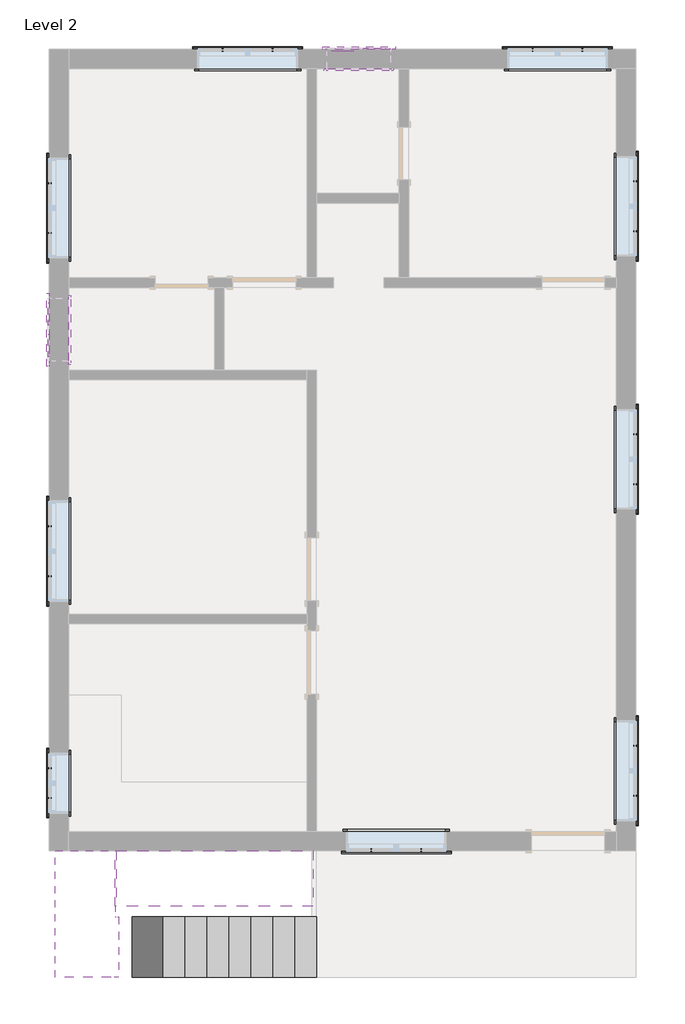
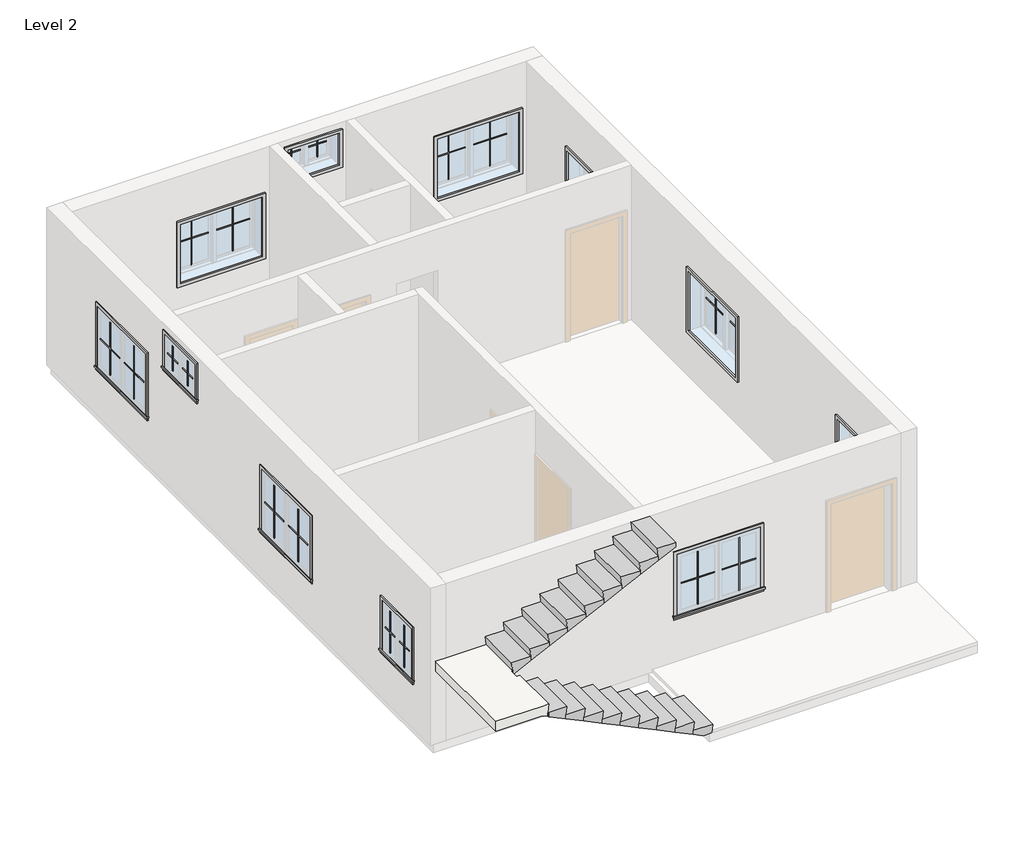
# One storey, part 2 of 2: 44 proxies, 2 stair flights, 1 slab.
"""IFC4 building model written with IfcOpenShell, lengths in millimetres."""

from ifc_helpers import new_model, si_unit, origin, place, context, project, spatial, faceted_brep, transform, mapped, element, save
from components import muntin_pattern_2x2_muntin_pattern_2x2_b3fe6957, muntin_pattern_2x2_muntin_pattern_2x2_3e0ecaf2, muntin_pattern_2x2_muntin_pattern_2x2_27d56209, muntin_pattern_2x2_muntin_pattern_2x2_bc89accc, muntin_pattern_2x2_muntin_pattern_2x2_1fe271a4, muntin_pattern_2x2_muntin_pattern_2x2_11ff06db, trim_window_exterior_flat_with_sill_41619996, trim_window_exterior_flat_with_sill_40e754a6, trim_window_exterior_flat_with_sill_f4abd27b, trim_window_interior_flat_picture_frame_51c85655, trim_window_interior_flat_picture_frame_6592d821, trim_window_interior_flat_picture_frame_286514af

model = new_model("IFC4")

# Units and contexts
model_context = context("Model", 3, world=origin())
ifc_project = project(units=[si_unit("LENGTHUNIT", "METRE", prefix="MILLI")], contexts=[model_context])

# Site, building, storey
site = spatial("IfcSite", under=ifc_project)
building = spatial("IfcBuilding", under=site)
storey = spatial("IfcBuildingStorey", under=building, Name="Level 2", Elevation=3048.0)

# Proxies
placement = place(None, origin())
muntin_pattern_2x2_muntin_pattern_2x2_shape = muntin_pattern_2x2_muntin_pattern_2x2_b3fe6957(model_context)
element("IfcBuildingElementProxy", 1, Name="Muntin Pattern_2x2 : Muntin Pattern_2x2", ObjectType="Muntin Pattern_2x2 : Muntin Pattern_2x2", at=placement, inside=storey, context=model_context, shape_type="MappedRepresentation", body=[
    mapped(muntin_pattern_2x2_muntin_pattern_2x2_shape, transform((-8839.6634077, -4303.4328663, 4032.25), x_axis=(0.0, 1.0, 0.0), y_axis=(-1.0, 0.0, 0.0), z_axis=(0.0, 0.0, 1.0))),
])
muntin_pattern_2x2_muntin_pattern_2x2_2_shape = muntin_pattern_2x2_muntin_pattern_2x2_3e0ecaf2(model_context)
element("IfcBuildingElementProxy", 2, Name="Muntin Pattern_2x2 : Muntin Pattern_2x2", ObjectType="Muntin Pattern_2x2 : Muntin Pattern_2x2", at=placement, inside=storey, context=model_context, shape_type="MappedRepresentation", body=[
    mapped(muntin_pattern_2x2_muntin_pattern_2x2_2_shape, transform((-8839.6634077, -3874.8078663, 4032.25), x_axis=(0.0, -1.0, 0.0), y_axis=(1.0, 0.0, 0.0), z_axis=(0.0, 0.0, 1.0))),
])
muntin_pattern_2x2_muntin_pattern_2x2_3_shape = muntin_pattern_2x2_muntin_pattern_2x2_27d56209(model_context)
element("IfcBuildingElementProxy", 3, Name="Muntin Pattern_2x2 : Muntin Pattern_2x2", ObjectType="Muntin Pattern_2x2 : Muntin Pattern_2x2", at=placement, inside=storey, context=model_context, shape_type="MappedRepresentation", body=[
    mapped(muntin_pattern_2x2_muntin_pattern_2x2_3_shape, transform((-8839.6634077, 2226.7657273, 5251.45), x_axis=(0.0, 1.0, 0.0), y_axis=(-1.0, 0.0, 0.0), z_axis=(0.0, 0.0, 1.0))),
])
element("IfcBuildingElementProxy", 4, Name="Muntin Pattern_2x2 : Muntin Pattern_2x2", ObjectType="Muntin Pattern_2x2 : Muntin Pattern_2x2", at=placement, inside=storey, context=model_context, shape_type="MappedRepresentation", body=[
    mapped(muntin_pattern_2x2_muntin_pattern_2x2_3_shape, transform((-4603.9220229, 6494.5392844, 5251.45), x_axis=(1.0, 0.0, 0.0), y_axis=(0.0, 1.0, 0.0), z_axis=(0.0, 0.0, 1.0))),
])
muntin_pattern_2x2_muntin_pattern_2x2_4_shape = muntin_pattern_2x2_muntin_pattern_2x2_bc89accc(model_context)
element("IfcBuildingElementProxy", 5, Name="Muntin Pattern_2x2 : Muntin Pattern_2x2", ObjectType="Muntin Pattern_2x2 : Muntin Pattern_2x2", at=placement, inside=storey, context=model_context, shape_type="MappedRepresentation", body=[
    mapped(muntin_pattern_2x2_muntin_pattern_2x2_4_shape, transform((-8839.6634077, 2680.7907273, 5251.45), x_axis=(0.0, -1.0, 0.0), y_axis=(1.0, 0.0, 0.0), z_axis=(0.0, 0.0, 1.0))),
])
element("IfcBuildingElementProxy", 6, Name="Muntin Pattern_2x2 : Muntin Pattern_2x2", ObjectType="Muntin Pattern_2x2 : Muntin Pattern_2x2", at=placement, inside=storey, context=model_context, shape_type="MappedRepresentation", body=[
    mapped(muntin_pattern_2x2_muntin_pattern_2x2_4_shape, transform((-4149.8970229, 6494.5392844, 5251.45), x_axis=(-1.0, 0.0, 0.0), y_axis=(0.0, -1.0, 0.0), z_axis=(0.0, 0.0, 1.0))),
])
muntin_pattern_2x2_muntin_pattern_2x2_5_shape = muntin_pattern_2x2_muntin_pattern_2x2_1fe271a4(model_context)
element("IfcBuildingElementProxy", 7, Name="Muntin Pattern_2x2 : Muntin Pattern_2x2", ObjectType="Muntin Pattern_2x2 : Muntin Pattern_2x2", at=placement, inside=storey, context=model_context, shape_type="MappedRepresentation", body=[
    mapped(muntin_pattern_2x2_muntin_pattern_2x2_5_shape, transform((-385.3035282, -3550.9578663, 4032.25), x_axis=(0.0, -1.0, 0.0), y_axis=(1.0, 0.0, 0.0), z_axis=(0.0, 0.0, 1.0))),
])
element("IfcBuildingElementProxy", 8, Name="Muntin Pattern_2x2 : Muntin Pattern_2x2", ObjectType="Muntin Pattern_2x2 : Muntin Pattern_2x2", at=placement, inside=storey, context=model_context, shape_type="MappedRepresentation", body=[
    mapped(muntin_pattern_2x2_muntin_pattern_2x2_5_shape, transform((-385.3035282, 944.8421337, 4032.25), x_axis=(0.0, -1.0, 0.0), y_axis=(1.0, 0.0, 0.0), z_axis=(0.0, 0.0, 1.0))),
])
element("IfcBuildingElementProxy", 9, Name="Muntin Pattern_2x2 : Muntin Pattern_2x2", ObjectType="Muntin Pattern_2x2 : Muntin Pattern_2x2", at=placement, inside=storey, context=model_context, shape_type="MappedRepresentation", body=[
    mapped(muntin_pattern_2x2_muntin_pattern_2x2_5_shape, transform((-385.3035282, 4597.1928819, 4032.25), x_axis=(0.0, -1.0, 0.0), y_axis=(1.0, 0.0, 0.0), z_axis=(0.0, 0.0, 1.0))),
])
element("IfcBuildingElementProxy", 10, Name="Muntin Pattern_2x2 : Muntin Pattern_2x2", ObjectType="Muntin Pattern_2x2 : Muntin Pattern_2x2", at=placement, inside=storey, context=model_context, shape_type="MappedRepresentation", body=[
    mapped(muntin_pattern_2x2_muntin_pattern_2x2_5_shape, transform((-1866.4410282, 6494.5392844, 4032.25), x_axis=(1.0, 0.0, 0.0), y_axis=(0.0, 1.0, 0.0), z_axis=(0.0, 0.0, 1.0))),
])
element("IfcBuildingElementProxy", 11, Name="Muntin Pattern_2x2 : Muntin Pattern_2x2", ObjectType="Muntin Pattern_2x2 : Muntin Pattern_2x2", at=placement, inside=storey, context=model_context, shape_type="MappedRepresentation", body=[
    mapped(muntin_pattern_2x2_muntin_pattern_2x2_5_shape, transform((-6342.5074828, 6494.5392844, 4032.25), x_axis=(1.0, 0.0, 0.0), y_axis=(0.0, 1.0, 0.0), z_axis=(0.0, 0.0, 1.0))),
])
element("IfcBuildingElementProxy", 12, Name="Muntin Pattern_2x2 : Muntin Pattern_2x2", ObjectType="Muntin Pattern_2x2 : Muntin Pattern_2x2", at=placement, inside=storey, context=model_context, shape_type="MappedRepresentation", body=[
    mapped(muntin_pattern_2x2_muntin_pattern_2x2_5_shape, transform((-8839.6634077, 3851.0678819, 4032.25), x_axis=(0.0, 1.0, 0.0), y_axis=(-1.0, 0.0, 0.0), z_axis=(0.0, 0.0, 1.0))),
])
element("IfcBuildingElementProxy", 13, Name="Muntin Pattern_2x2 : Muntin Pattern_2x2", ObjectType="Muntin Pattern_2x2 : Muntin Pattern_2x2", at=placement, inside=storey, context=model_context, shape_type="MappedRepresentation", body=[
    mapped(muntin_pattern_2x2_muntin_pattern_2x2_5_shape, transform((-8839.6634077, -1101.0873314, 4032.25), x_axis=(0.0, 1.0, 0.0), y_axis=(-1.0, 0.0, 0.0), z_axis=(0.0, 0.0, 1.0))),
])
element("IfcBuildingElementProxy", 14, Name="Muntin Pattern_2x2 : Muntin Pattern_2x2", ObjectType="Muntin Pattern_2x2 : Muntin Pattern_2x2", at=placement, inside=storey, context=model_context, shape_type="MappedRepresentation", body=[
    mapped(muntin_pattern_2x2_muntin_pattern_2x2_5_shape, transform((-3475.4824828, -5057.4953663, 4032.25), x_axis=(-1.0, 0.0, 0.0), y_axis=(0.0, -1.0, 0.0), z_axis=(0.0, 0.0, 1.0))),
])
muntin_pattern_2x2_muntin_pattern_2x2_6_shape = muntin_pattern_2x2_muntin_pattern_2x2_11ff06db(model_context)
element("IfcBuildingElementProxy", 15, Name="Muntin Pattern_2x2 : Muntin Pattern_2x2", ObjectType="Muntin Pattern_2x2 : Muntin Pattern_2x2", at=placement, inside=storey, context=model_context, shape_type="MappedRepresentation", body=[
    mapped(muntin_pattern_2x2_muntin_pattern_2x2_6_shape, transform((-385.3035282, -4271.6828663, 4032.25), x_axis=(0.0, 1.0, 0.0), y_axis=(-1.0, 0.0, 0.0), z_axis=(0.0, 0.0, 1.0))),
])
element("IfcBuildingElementProxy", 16, Name="Muntin Pattern_2x2 : Muntin Pattern_2x2", ObjectType="Muntin Pattern_2x2 : Muntin Pattern_2x2", at=placement, inside=storey, context=model_context, shape_type="MappedRepresentation", body=[
    mapped(muntin_pattern_2x2_muntin_pattern_2x2_6_shape, transform((-385.3035282, 224.1171337, 4032.25), x_axis=(0.0, 1.0, 0.0), y_axis=(-1.0, 0.0, 0.0), z_axis=(0.0, 0.0, 1.0))),
])
element("IfcBuildingElementProxy", 17, Name="Muntin Pattern_2x2 : Muntin Pattern_2x2", ObjectType="Muntin Pattern_2x2 : Muntin Pattern_2x2", at=placement, inside=storey, context=model_context, shape_type="MappedRepresentation", body=[
    mapped(muntin_pattern_2x2_muntin_pattern_2x2_6_shape, transform((-385.3035282, 3876.4678819, 4032.25), x_axis=(0.0, 1.0, 0.0), y_axis=(-1.0, 0.0, 0.0), z_axis=(0.0, 0.0, 1.0))),
])
element("IfcBuildingElementProxy", 18, Name="Muntin Pattern_2x2 : Muntin Pattern_2x2", ObjectType="Muntin Pattern_2x2 : Muntin Pattern_2x2", at=placement, inside=storey, context=model_context, shape_type="MappedRepresentation", body=[
    mapped(muntin_pattern_2x2_muntin_pattern_2x2_6_shape, transform((-1145.7160282, 6494.5392844, 4032.25), x_axis=(-1.0, 0.0, 0.0), y_axis=(0.0, -1.0, 0.0), z_axis=(0.0, 0.0, 1.0))),
])
element("IfcBuildingElementProxy", 19, Name="Muntin Pattern_2x2 : Muntin Pattern_2x2", ObjectType="Muntin Pattern_2x2 : Muntin Pattern_2x2", at=placement, inside=storey, context=model_context, shape_type="MappedRepresentation", body=[
    mapped(muntin_pattern_2x2_muntin_pattern_2x2_6_shape, transform((-5621.7824828, 6494.5392844, 4032.25), x_axis=(-1.0, 0.0, 0.0), y_axis=(0.0, -1.0, 0.0), z_axis=(0.0, 0.0, 1.0))),
])
element("IfcBuildingElementProxy", 20, Name="Muntin Pattern_2x2 : Muntin Pattern_2x2", ObjectType="Muntin Pattern_2x2 : Muntin Pattern_2x2", at=placement, inside=storey, context=model_context, shape_type="MappedRepresentation", body=[
    mapped(muntin_pattern_2x2_muntin_pattern_2x2_6_shape, transform((-8839.6634077, 4571.7928819, 4032.25), x_axis=(0.0, -1.0, 0.0), y_axis=(1.0, 0.0, 0.0), z_axis=(0.0, 0.0, 1.0))),
])
element("IfcBuildingElementProxy", 21, Name="Muntin Pattern_2x2 : Muntin Pattern_2x2", ObjectType="Muntin Pattern_2x2 : Muntin Pattern_2x2", at=placement, inside=storey, context=model_context, shape_type="MappedRepresentation", body=[
    mapped(muntin_pattern_2x2_muntin_pattern_2x2_6_shape, transform((-8839.6634077, -380.3623314, 4032.25), x_axis=(0.0, -1.0, 0.0), y_axis=(1.0, 0.0, 0.0), z_axis=(0.0, 0.0, 1.0))),
])
element("IfcBuildingElementProxy", 22, Name="Muntin Pattern_2x2 : Muntin Pattern_2x2", ObjectType="Muntin Pattern_2x2 : Muntin Pattern_2x2", at=placement, inside=storey, context=model_context, shape_type="MappedRepresentation", body=[
    mapped(muntin_pattern_2x2_muntin_pattern_2x2_6_shape, transform((-4196.2074828, -5057.4953663, 4032.25), x_axis=(1.0, 0.0, 0.0), y_axis=(0.0, 1.0, 0.0), z_axis=(0.0, 0.0, 1.0))),
])
trim_window_exterior_flat_with_sill_shape = trim_window_exterior_flat_with_sill_41619996(model_context)
element("IfcBuildingElementProxy", 23, Name="Trim-Window-Exterior-Flat : with Sill", ObjectType="Trim-Window-Exterior-Flat : with Sill", at=placement, inside=storey, context=model_context, shape_type="MappedRepresentation", body=[
    mapped(trim_window_exterior_flat_with_sill_shape, transform((-8849.1884077, -4089.1203663, 4876.8), x_axis=(0.0, -1.0, 0.0), y_axis=(0.0, 0.0, 1.0), z_axis=(-1.0, 0.0, 0.0))),
])
trim_window_exterior_flat_with_sill_2_shape = trim_window_exterior_flat_with_sill_40e754a6(model_context)
element("IfcBuildingElementProxy", 24, Name="Trim-Window-Exterior-Flat : with Sill", ObjectType="Trim-Window-Exterior-Flat : with Sill", at=placement, inside=storey, context=model_context, shape_type="MappedRepresentation", body=[
    mapped(trim_window_exterior_flat_with_sill_2_shape, transform((-8849.1884077, 2453.7782273, 5791.2), x_axis=(0.0, -1.0, 0.0), y_axis=(0.0, 0.0, 1.0), z_axis=(-1.0, 0.0, 0.0))),
])
element("IfcBuildingElementProxy", 25, Name="Trim-Window-Exterior-Flat : with Sill", ObjectType="Trim-Window-Exterior-Flat : with Sill", at=placement, inside=storey, context=model_context, shape_type="MappedRepresentation", body=[
    mapped(trim_window_exterior_flat_with_sill_2_shape, transform((-4376.9095229, 6504.0642844, 5791.2), x_axis=(-1.0, 0.0, 0.0), y_axis=(0.0, 0.0, 1.0), z_axis=(0.0, 1.0, 0.0))),
])
trim_window_exterior_flat_with_sill_3_shape = trim_window_exterior_flat_with_sill_f4abd27b(model_context)
element("IfcBuildingElementProxy", 26, Name="Trim-Window-Exterior-Flat : with Sill", ObjectType="Trim-Window-Exterior-Flat : with Sill", at=placement, inside=storey, context=model_context, shape_type="MappedRepresentation", body=[
    mapped(trim_window_exterior_flat_with_sill_3_shape, transform((-375.7785282, -3911.3203663, 5080.0), x_axis=(0.0, 1.0, 0.0), y_axis=(0.0, 0.0, 1.0), z_axis=(1.0, 0.0, 0.0))),
])
element("IfcBuildingElementProxy", 27, Name="Trim-Window-Exterior-Flat : with Sill", ObjectType="Trim-Window-Exterior-Flat : with Sill", at=placement, inside=storey, context=model_context, shape_type="MappedRepresentation", body=[
    mapped(trim_window_exterior_flat_with_sill_3_shape, transform((-375.7785282, 584.4796337, 5080.0), x_axis=(0.0, 1.0, 0.0), y_axis=(0.0, 0.0, 1.0), z_axis=(1.0, 0.0, 0.0))),
])
element("IfcBuildingElementProxy", 28, Name="Trim-Window-Exterior-Flat : with Sill", ObjectType="Trim-Window-Exterior-Flat : with Sill", at=placement, inside=storey, context=model_context, shape_type="MappedRepresentation", body=[
    mapped(trim_window_exterior_flat_with_sill_3_shape, transform((-375.7785282, 4236.8303819, 5080.0), x_axis=(0.0, 1.0, 0.0), y_axis=(0.0, 0.0, 1.0), z_axis=(1.0, 0.0, 0.0))),
])
element("IfcBuildingElementProxy", 29, Name="Trim-Window-Exterior-Flat : with Sill", ObjectType="Trim-Window-Exterior-Flat : with Sill", at=placement, inside=storey, context=model_context, shape_type="MappedRepresentation", body=[
    mapped(trim_window_exterior_flat_with_sill_3_shape, transform((-1506.0785282, 6504.0642844, 5080.0), x_axis=(-1.0, 0.0, 0.0), y_axis=(0.0, 0.0, 1.0), z_axis=(0.0, 1.0, 0.0))),
])
element("IfcBuildingElementProxy", 30, Name="Trim-Window-Exterior-Flat : with Sill", ObjectType="Trim-Window-Exterior-Flat : with Sill", at=placement, inside=storey, context=model_context, shape_type="MappedRepresentation", body=[
    mapped(trim_window_exterior_flat_with_sill_3_shape, transform((-5982.1449828, 6504.0642844, 5080.0), x_axis=(-1.0, 0.0, 0.0), y_axis=(0.0, 0.0, 1.0), z_axis=(0.0, 1.0, 0.0))),
])
element("IfcBuildingElementProxy", 31, Name="Trim-Window-Exterior-Flat : with Sill", ObjectType="Trim-Window-Exterior-Flat : with Sill", at=placement, inside=storey, context=model_context, shape_type="MappedRepresentation", body=[
    mapped(trim_window_exterior_flat_with_sill_3_shape, transform((-8849.1884077, 4211.4303819, 5080.0), x_axis=(0.0, -1.0, 0.0), y_axis=(0.0, 0.0, 1.0), z_axis=(-1.0, 0.0, 0.0))),
])
element("IfcBuildingElementProxy", 32, Name="Trim-Window-Exterior-Flat : with Sill", ObjectType="Trim-Window-Exterior-Flat : with Sill", at=placement, inside=storey, context=model_context, shape_type="MappedRepresentation", body=[
    mapped(trim_window_exterior_flat_with_sill_3_shape, transform((-8849.1884077, -740.7248314, 5080.0), x_axis=(0.0, -1.0, 0.0), y_axis=(0.0, 0.0, 1.0), z_axis=(-1.0, 0.0, 0.0))),
])
element("IfcBuildingElementProxy", 33, Name="Trim-Window-Exterior-Flat : with Sill", ObjectType="Trim-Window-Exterior-Flat : with Sill", at=placement, inside=storey, context=model_context, shape_type="MappedRepresentation", body=[
    mapped(trim_window_exterior_flat_with_sill_3_shape, transform((-3835.8449828, -5067.0203663, 5080.0), x_axis=(1.0, 0.0, 0.0), y_axis=(0.0, 0.0, 1.0), z_axis=(0.0, -1.0, 0.0))),
])
trim_window_interior_flat_picture_frame_shape = trim_window_interior_flat_picture_frame_51c85655(model_context)
element("IfcBuildingElementProxy", 34, Name="Trim-Window-Interior-Flat : Picture Frame", ObjectType="Trim-Window-Interior-Flat : Picture Frame", at=placement, inside=storey, context=model_context, shape_type="MappedRepresentation", body=[
    mapped(trim_window_interior_flat_picture_frame_shape, transform((-8569.7884077, -4089.1203663, 4876.8), x_axis=(0.0, 1.0, 0.0), y_axis=(0.0, 0.0, 1.0), z_axis=(1.0, 0.0, 0.0))),
])
trim_window_interior_flat_picture_frame_2_shape = trim_window_interior_flat_picture_frame_6592d821(model_context)
element("IfcBuildingElementProxy", 35, Name="Trim-Window-Interior-Flat : Picture Frame", ObjectType="Trim-Window-Interior-Flat : Picture Frame", at=placement, inside=storey, context=model_context, shape_type="MappedRepresentation", body=[
    mapped(trim_window_interior_flat_picture_frame_2_shape, transform((-8569.7884077, 2453.7782273, 5791.2), x_axis=(0.0, 1.0, 0.0), y_axis=(0.0, 0.0, 1.0), z_axis=(1.0, 0.0, 0.0))),
])
element("IfcBuildingElementProxy", 36, Name="Trim-Window-Interior-Flat : Picture Frame", ObjectType="Trim-Window-Interior-Flat : Picture Frame", at=placement, inside=storey, context=model_context, shape_type="MappedRepresentation", body=[
    mapped(trim_window_interior_flat_picture_frame_2_shape, transform((-4376.9095229, 6224.6642844, 5791.2), x_axis=(1.0, 0.0, 0.0), y_axis=(0.0, 0.0, 1.0), z_axis=(0.0, -1.0, 0.0))),
])
trim_window_interior_flat_picture_frame_3_shape = trim_window_interior_flat_picture_frame_286514af(model_context)
element("IfcBuildingElementProxy", 37, Name="Trim-Window-Interior-Flat : Picture Frame", ObjectType="Trim-Window-Interior-Flat : Picture Frame", at=placement, inside=storey, context=model_context, shape_type="MappedRepresentation", body=[
    mapped(trim_window_interior_flat_picture_frame_3_shape, transform((-655.1785282, -3911.3203663, 5080.0), x_axis=(0.0, -1.0, 0.0), y_axis=(0.0, 0.0, 1.0), z_axis=(-1.0, 0.0, 0.0))),
])
element("IfcBuildingElementProxy", 38, Name="Trim-Window-Interior-Flat : Picture Frame", ObjectType="Trim-Window-Interior-Flat : Picture Frame", at=placement, inside=storey, context=model_context, shape_type="MappedRepresentation", body=[
    mapped(trim_window_interior_flat_picture_frame_3_shape, transform((-655.1785282, 584.4796337, 5080.0), x_axis=(0.0, -1.0, 0.0), y_axis=(0.0, 0.0, 1.0), z_axis=(-1.0, 0.0, 0.0))),
])
element("IfcBuildingElementProxy", 39, Name="Trim-Window-Interior-Flat : Picture Frame", ObjectType="Trim-Window-Interior-Flat : Picture Frame", at=placement, inside=storey, context=model_context, shape_type="MappedRepresentation", body=[
    mapped(trim_window_interior_flat_picture_frame_3_shape, transform((-655.1785282, 4236.8303819, 5080.0), x_axis=(0.0, -1.0, 0.0), y_axis=(0.0, 0.0, 1.0), z_axis=(-1.0, 0.0, 0.0))),
])
element("IfcBuildingElementProxy", 40, Name="Trim-Window-Interior-Flat : Picture Frame", ObjectType="Trim-Window-Interior-Flat : Picture Frame", at=placement, inside=storey, context=model_context, shape_type="MappedRepresentation", body=[
    mapped(trim_window_interior_flat_picture_frame_3_shape, transform((-1506.0785282, 6224.6642844, 5080.0), x_axis=(1.0, 0.0, 0.0), y_axis=(0.0, 0.0, 1.0), z_axis=(0.0, -1.0, 0.0))),
])
element("IfcBuildingElementProxy", 41, Name="Trim-Window-Interior-Flat : Picture Frame", ObjectType="Trim-Window-Interior-Flat : Picture Frame", at=placement, inside=storey, context=model_context, shape_type="MappedRepresentation", body=[
    mapped(trim_window_interior_flat_picture_frame_3_shape, transform((-5982.1449828, 6224.6642844, 5080.0), x_axis=(1.0, 0.0, 0.0), y_axis=(0.0, 0.0, 1.0), z_axis=(0.0, -1.0, 0.0))),
])
element("IfcBuildingElementProxy", 42, Name="Trim-Window-Interior-Flat : Picture Frame", ObjectType="Trim-Window-Interior-Flat : Picture Frame", at=placement, inside=storey, context=model_context, shape_type="MappedRepresentation", body=[
    mapped(trim_window_interior_flat_picture_frame_3_shape, transform((-8569.7884077, 4211.4303819, 5080.0), x_axis=(0.0, 1.0, 0.0), y_axis=(0.0, 0.0, 1.0), z_axis=(1.0, 0.0, 0.0))),
])
element("IfcBuildingElementProxy", 43, Name="Trim-Window-Interior-Flat : Picture Frame", ObjectType="Trim-Window-Interior-Flat : Picture Frame", at=placement, inside=storey, context=model_context, shape_type="MappedRepresentation", body=[
    mapped(trim_window_interior_flat_picture_frame_3_shape, transform((-8569.7884077, -740.7248314, 5080.0), x_axis=(0.0, 1.0, 0.0), y_axis=(0.0, 0.0, 1.0), z_axis=(1.0, 0.0, 0.0))),
])
element("IfcBuildingElementProxy", 44, Name="Trim-Window-Interior-Flat : Picture Frame", ObjectType="Trim-Window-Interior-Flat : Picture Frame", at=placement, inside=storey, context=model_context, shape_type="MappedRepresentation", body=[
    mapped(trim_window_interior_flat_picture_frame_3_shape, transform((-3835.8449828, -4787.6203663, 5080.0), x_axis=(-1.0, 0.0, 0.0), y_axis=(0.0, 0.0, 1.0), z_axis=(0.0, 1.0, 0.0))),
])

# Slab
element("IfcSlab", 45, ObjectType="7\" Thickness", at=placement, inside=storey, context=model_context, shape_type="Brep", body=[
    faceted_brep([(-7896.6884077, -6018.2039507, 4572.0), (-7896.6884077, -5868.2058051, 4572.0), (-7877.6384077, -5868.2058051, 4572.0), (-7877.6384077, -5067.0203663, 4572.0), (-7896.6884077, -5067.0203663, 4572.0), (-8101.3126638, -5067.0203663, 4572.0), (-8760.2884077, -5067.0203663, 4572.0), (-8760.2884077, -6894.0922127, 4572.0), (-7955.5707267, -6894.0922127, 4572.0), (-7842.6949828, -6894.0922127, 4572.0), (-7842.6949828, -6018.2039507, 4572.0), (-7861.7449828, -6018.2039507, 4419.6), (-7861.7449828, -6894.0922127, 4419.6), (-7861.7449828, -6894.0922127, 4349.1636429), (-7861.7449828, -6018.2039507, 4349.1636429), (-7955.5707267, -6018.2039507, 4394.2), (-7896.6884077, -6018.2039507, 4394.2), (-7896.6884077, -5868.2058051, 4394.2), (-7896.6884077, -5868.2058051, 4492.4196429), (-7877.6384077, -5868.2058051, 4501.5636429), (-7877.6384077, -5067.0203663, 4501.5636429), (-7896.6884077, -5067.0203663, 4492.4196429), (-8101.3126638, -5067.0203663, 4394.2), (-8760.2884077, -5067.0203663, 4394.2), (-8760.2884077, -6894.0922127, 4394.2), (-7955.5707267, -6894.0922127, 4394.2), (-8101.3126638, -5868.2058051, 4394.2)], [[[0, 1, 2, 3, 4, 5, 6, 7, 8, 9, 10]], [[11, 12, 13, 14]], [[0, 10, 11, 14, 15, 16]], [[1, 0, 16, 17, 18]], [[2, 1, 18, 19]], [[3, 2, 19, 20]], [[4, 3, 20, 21]], [[4, 21, 22, 23, 6, 5]], [[7, 6, 23, 24]], [[12, 9, 8, 7, 24, 25, 13]], [[10, 9, 12, 11]], [[26, 17, 16, 15, 25, 24, 23, 22]], [[17, 26, 18]], [[25, 15, 14, 13]], [[26, 22, 21, 20, 19, 18]]]),
])

# Stair flights
element("IfcStairFlight", 46, ObjectType="3/4\" Nosing", at=placement, inside=storey, context=model_context, shape_type="Brep", body=[
    faceted_brep([(-4985.1949828, -6894.0922127, 3200.4), (-4985.1949828, -6018.2039507, 3200.4), (-5321.7449828, -6018.2039507, 3200.4), (-5321.7449828, -6894.0922127, 3200.4), (-5321.7449828, -6894.0922127, 3129.9636429), (-5150.9873934, -6894.0922127, 3048.0), (-5004.2449828, -6894.0922127, 3048.0), (-5004.2449828, -6018.2039507, 3048.0), (-5150.9873934, -6018.2039507, 3048.0), (-5321.7449828, -6018.2039507, 3129.9636429), (-5302.6949828, -6894.0922127, 3352.8), (-5302.6949828, -6018.2039507, 3352.8), (-5639.2449828, -6018.2039507, 3352.8), (-5639.2449828, -6894.0922127, 3352.8), (-5639.2449828, -6894.0922127, 3282.3636429), (-5639.2449828, -6018.2039507, 3282.3636429), (-5620.1949828, -6894.0922127, 3505.2), (-5620.1949828, -6018.2039507, 3505.2), (-5956.7449828, -6018.2039507, 3505.2), (-5956.7449828, -6894.0922127, 3505.2), (-5956.7449828, -6894.0922127, 3434.7636429), (-5956.7449828, -6018.2039507, 3434.7636429), (-5937.6949828, -6894.0922127, 3657.6), (-5937.6949828, -6018.2039507, 3657.6), (-6274.2449828, -6018.2039507, 3657.6), (-6274.2449828, -6894.0922127, 3657.6), (-6274.2449828, -6894.0922127, 3587.1636429), (-6274.2449828, -6018.2039507, 3587.1636429), (-6255.1949828, -6894.0922127, 3810.0), (-6255.1949828, -6018.2039507, 3810.0), (-6591.7449828, -6018.2039507, 3810.0), (-6591.7449828, -6894.0922127, 3810.0), (-6591.7449828, -6894.0922127, 3739.5636429), (-6591.7449828, -6018.2039507, 3739.5636429), (-6572.6949828, -6894.0922127, 3962.4), (-6572.6949828, -6018.2039507, 3962.4), (-6909.2449828, -6018.2039507, 3962.4), (-6909.2449828, -6894.0922127, 3962.4), (-6909.2449828, -6894.0922127, 3891.9636429), (-6909.2449828, -6018.2039507, 3891.9636429), (-6890.1949828, -6894.0922127, 4114.8), (-6890.1949828, -6018.2039507, 4114.8), (-7226.7449828, -6018.2039507, 4114.8), (-7226.7449828, -6894.0922127, 4114.8), (-7226.7449828, -6894.0922127, 4044.3636429), (-7226.7449828, -6018.2039507, 4044.3636429), (-7207.6949828, -6894.0922127, 4267.2), (-7207.6949828, -6018.2039507, 4267.2), (-7544.2449828, -6018.2039507, 4267.2), (-7544.2449828, -6894.0922127, 4267.2), (-7544.2449828, -6894.0922127, 4196.7636429), (-7544.2449828, -6018.2039507, 4196.7636429), (-7861.7449828, -6894.0922127, 4419.6), (-7842.6949828, -6894.0922127, 4419.6), (-7525.1949828, -6894.0922127, 4419.6), (-7525.1949828, -6018.2039507, 4419.6), (-7842.6949828, -6018.2039507, 4419.6), (-7861.7449828, -6018.2039507, 4419.6), (-7861.7449828, -6894.0922127, 4349.1636429), (-7842.6949828, -6894.0922127, 4340.0196429), (-7842.6949828, -6018.2039507, 4340.0196429), (-7861.7449828, -6018.2039507, 4349.1636429)], [[[0, 1, 2, 3]], [[0, 3, 4, 5, 6]], [[2, 1, 7, 8, 9]], [[10, 11, 12, 13]], [[10, 13, 14, 4, 3]], [[12, 11, 2, 9, 15]], [[16, 17, 18, 19]], [[16, 19, 20, 14, 13]], [[18, 17, 12, 15, 21]], [[22, 23, 24, 25]], [[22, 25, 26, 20, 19]], [[24, 23, 18, 21, 27]], [[28, 29, 30, 31]], [[28, 31, 32, 26, 25]], [[30, 29, 24, 27, 33]], [[34, 35, 36, 37]], [[34, 37, 38, 32, 31]], [[36, 35, 30, 33, 39]], [[40, 41, 42, 43]], [[40, 43, 44, 38, 37]], [[42, 41, 36, 39, 45]], [[46, 47, 48, 49]], [[46, 49, 50, 44, 43]], [[48, 47, 42, 45, 51]], [[52, 53, 54, 55, 56, 57]], [[53, 52, 58, 59]], [[54, 53, 59, 50, 49]], [[56, 55, 48, 51, 60]], [[57, 56, 60, 61]], [[52, 57, 61, 58]], [[1, 0, 6, 7]], [[3, 2, 11, 10]], [[13, 12, 17, 16]], [[19, 18, 23, 22]], [[25, 24, 29, 28]], [[31, 30, 35, 34]], [[37, 36, 41, 40]], [[43, 42, 47, 46]], [[49, 48, 55, 54]], [[7, 6, 5, 8]], [[8, 5, 4, 14, 20, 26, 32, 38, 44, 50, 59, 58, 61, 60, 51, 45, 39, 33, 27, 21, 15, 9]]]),
])
element("IfcStairFlight", 47, ObjectType="3/4\" Nosing", at=placement, inside=storey, context=model_context, shape_type="Brep", body=[
    faceted_brep([(-7896.6884077, -5067.0203663, 4724.4), (-7896.6884077, -5868.2058051, 4724.4), (-7560.1384077, -5868.2058051, 4724.4), (-7560.1384077, -5067.0203663, 4724.4), (-7560.1384077, -5067.0203663, 4653.9636429), (-7877.6384077, -5067.0203663, 4501.5636429), (-7877.6384077, -5067.0203663, 4572.0), (-7877.6384077, -5868.2058051, 4572.0), (-7877.6384077, -5868.2058051, 4501.5636429), (-7560.1384077, -5868.2058051, 4653.9636429), (-7579.1884077, -5067.0203663, 4876.8), (-7579.1884077, -5868.2058051, 4876.8), (-7242.6384077, -5868.2058051, 4876.8), (-7242.6384077, -5067.0203663, 4876.8), (-7242.6384077, -5067.0203663, 4806.3636429), (-7242.6384077, -5868.2058051, 4806.3636429), (-7261.6884077, -5067.0203663, 5029.2), (-7261.6884077, -5868.2058051, 5029.2), (-6925.1384077, -5868.2058051, 5029.2), (-6925.1384077, -5067.0203663, 5029.2), (-6925.1384077, -5067.0203663, 4958.7636429), (-6925.1384077, -5868.2058051, 4958.7636429), (-6944.1884077, -5067.0203663, 5181.6), (-6944.1884077, -5868.2058051, 5181.6), (-6607.6384077, -5868.2058051, 5181.6), (-6607.6384077, -5067.0203663, 5181.6), (-6607.6384077, -5067.0203663, 5111.1636429), (-6607.6384077, -5868.2058051, 5111.1636429), (-6626.6884077, -5067.0203663, 5334.0), (-6626.6884077, -5868.2058051, 5334.0), (-6290.1384077, -5868.2058051, 5334.0), (-6290.1384077, -5067.0203663, 5334.0), (-6290.1384077, -5067.0203663, 5263.5636429), (-6290.1384077, -5868.2058051, 5263.5636429), (-6309.1884077, -5067.0203663, 5486.4), (-6309.1884077, -5868.2058051, 5486.4), (-5972.6384077, -5868.2058051, 5486.4), (-5972.6384077, -5067.0203663, 5486.4), (-5972.6384077, -5067.0203663, 5415.9636429), (-5972.6384077, -5868.2058051, 5415.9636429), (-5991.6884077, -5067.0203663, 5638.8), (-5991.6884077, -5868.2058051, 5638.8), (-5655.1384077, -5868.2058051, 5638.8), (-5655.1384077, -5067.0203663, 5638.8), (-5655.1384077, -5067.0203663, 5568.3636429), (-5655.1384077, -5868.2058051, 5568.3636429), (-5674.1884077, -5067.0203663, 5791.2), (-5674.1884077, -5868.2058051, 5791.2), (-5337.6384077, -5868.2058051, 5791.2), (-5337.6384077, -5067.0203663, 5791.2), (-5337.6384077, -5067.0203663, 5720.7636429), (-5337.6384077, -5868.2058051, 5720.7636429), (-5356.6884077, -5067.0203663, 5943.6), (-5356.6884077, -5868.2058051, 5943.6), (-5039.1884077, -5868.2058051, 5943.6), (-5039.1884077, -5067.0203663, 5943.6), (-5039.1884077, -5067.0203663, 5864.0196429), (-5039.1884077, -5868.2058051, 5864.0196429)], [[[0, 1, 2, 3]], [[0, 3, 4, 5, 6]], [[7, 6, 5, 8]], [[2, 1, 7, 8, 9]], [[10, 11, 12, 13]], [[10, 13, 14, 4, 3]], [[12, 11, 2, 9, 15]], [[16, 17, 18, 19]], [[16, 19, 20, 14, 13]], [[18, 17, 12, 15, 21]], [[22, 23, 24, 25]], [[22, 25, 26, 20, 19]], [[24, 23, 18, 21, 27]], [[28, 29, 30, 31]], [[28, 31, 32, 26, 25]], [[30, 29, 24, 27, 33]], [[34, 35, 36, 37]], [[34, 37, 38, 32, 31]], [[36, 35, 30, 33, 39]], [[40, 41, 42, 43]], [[40, 43, 44, 38, 37]], [[42, 41, 36, 39, 45]], [[46, 47, 48, 49]], [[46, 49, 50, 44, 43]], [[48, 47, 42, 45, 51]], [[1, 0, 6, 7]], [[11, 10, 3, 2]], [[17, 16, 13, 12]], [[23, 22, 19, 18]], [[29, 28, 25, 24]], [[35, 34, 31, 30]], [[41, 40, 37, 36]], [[47, 46, 43, 42]], [[52, 53, 54, 55]], [[52, 55, 56, 50, 49]], [[54, 53, 48, 51, 57]], [[55, 54, 57, 56]], [[53, 52, 49, 48]], [[5, 4, 14, 20, 26, 32, 38, 44, 50, 56, 57, 51, 45, 39, 33, 27, 21, 15, 9, 8]]]),
])

save(model, "model.ifc")

# Revit data of these elements
# Type "Muntin Pattern_2x2 : Muntin Pattern_2x2"
#   Width [instance default] = 48"
#   Thickness = 0.5"
#   Height [instance default] = 48"
#   Distance = 0.75"
#   Interior Material [instance default] = none
#   Exterior Material [instance default] = none
#   Default Elevation = 0
# Type "Trim-Window-Exterior-Flat : with Sill"
#   Trim Width = 2.25"
#   Trim Thickness_Picture Frame = 1.25"
#   Trim Thickness_with Sill = 0.75"
#   Sill Thickness = 1.25"
#   Opening Width [instance default] = 24"
#   Opening Height [instance default] = 36"
#   Default Elevation = 48"
#   Sill = yes
#   Picture Frame = no
#   Trim Material [instance default] = none
# Type "Trim-Window-Interior-Flat : Picture Frame"
#   Trim Thickness_Picture Frame = 1.25"
#   Trim Width = 2.25"
#   Trim Thickness_with Sill = 0.75"
#   Sill Thickness = 1.25"
#   Opening Width [instance default] = 24"
#   Opening Height [instance default] = 36"
#   Default Elevation = 48"
#   Sill = no
#   Picture Frame = yes
#   Trim Material [instance default] = none
# Elements 1, 2 (IfcBuildingElementProxy, "Muntin Pattern_2x2 : Muntin Pattern_2x2")
#   Width = 11.625"
#   Height = 30.5"
#   Interior Material = Wood - Stained
#   Exterior Material = Clad - White
#   Phase Created = New Construction
#   Materials on its faces: "Clad - White", "Wood - Stained"
# Elements 3, 4, 5, 6 (IfcBuildingElementProxy, "Muntin Pattern_2x2 : Muntin Pattern_2x2")
#   Width = 12.625"
#   Height = 18.5"
#   Interior Material = Wood - Stained
#   Exterior Material = Clad - White
#   Phase Created = New Construction
#   Materials on its faces: "Clad - White", "Wood - Stained"
# Elements 7, 8, 9, 10, 11, 12, 13, 14, 15, 16, 17, 18, 19, 20, 21, 22 (IfcBuildingElementProxy, "Muntin Pattern_2x2 : Muntin Pattern_2x2")
#   Width = 23.125"
#   Height = 38.5"
#   Interior Material = Wood - Stained
#   Exterior Material = Clad - White
#   Phase Created = New Construction
#   Materials on its faces: "Clad - White", "Wood - Stained"
# Element 23 (IfcBuildingElementProxy, "Trim-Window-Exterior-Flat : with Sill")
#   Opening Width = 34"
#   Opening Height = 36"
#   Trim Material = Clad - White
#   Phase Created = New Construction
#   Materials on its faces: "Clad - White"
# Elements 24, 25 (IfcBuildingElementProxy, "Trim-Window-Exterior-Flat : with Sill")
#   Opening Width = 36"
#   Opening Height = 24"
#   Trim Material = Clad - White
#   Phase Created = New Construction
#   Materials on its faces: "Clad - White"
# Elements 26, 27, 28, 29, 30, 31, 32, 33 (IfcBuildingElementProxy, "Trim-Window-Exterior-Flat : with Sill")
#   Opening Width = 57"
#   Opening Height = 44"
#   Trim Material = Clad - White
#   Phase Created = New Construction
#   Materials on its faces: "Clad - White"
# Element 34 (IfcBuildingElementProxy, "Trim-Window-Interior-Flat : Picture Frame")
#   Opening Width = 34"
#   Opening Height = 36"
#   Trim Material = Wood - Stained
#   Phase Created = New Construction
#   Materials on its faces: "Wood - Stained"
# Elements 35, 36 (IfcBuildingElementProxy, "Trim-Window-Interior-Flat : Picture Frame")
#   Opening Width = 36"
#   Opening Height = 24"
#   Trim Material = Wood - Stained
#   Phase Created = New Construction
#   Materials on its faces: "Wood - Stained"
# Elements 37, 38, 39, 40, 41, 42, 43, 44 (IfcBuildingElementProxy, "Trim-Window-Interior-Flat : Picture Frame")
#   Opening Width = 57"
#   Opening Height = 44"
#   Trim Material = Wood - Stained
#   Phase Created = New Construction
#   Materials on its faces: "Wood - Stained"
# Element 45 (IfcSlab, "7\" Thickness")
#   Phase Created = New Construction
#   Materials on its faces: "Concrete, Cast-in-Place gray"
# Elements 46, 47 (IfcStairFlight, "3/4\" Nosing")
#   Phase Created = New Construction
#   Materials on its faces: "Concrete, Cast-in-Place gray"
# Materials
#   "Clad - White": class "Wood", colour RGB 242 242 238, transparency 0, Cost = 0
#   "Wood - Stained": class "Wood", colour RGB 224 178 126, transparency 0, Cost = 0
#   "Concrete, Cast-in-Place gray": class "Concrete", colour RGB 192 192 192, transparency 0, Description = "Cast-in-place concrete", Cost = 0
